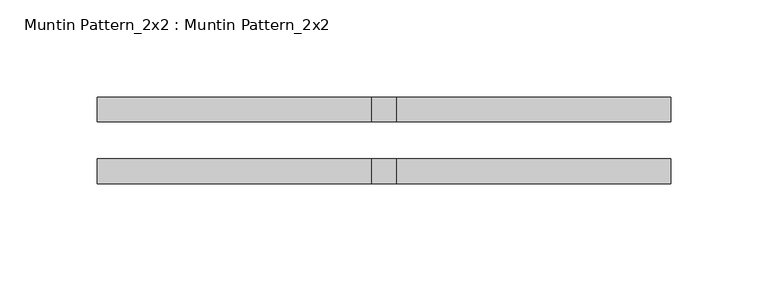
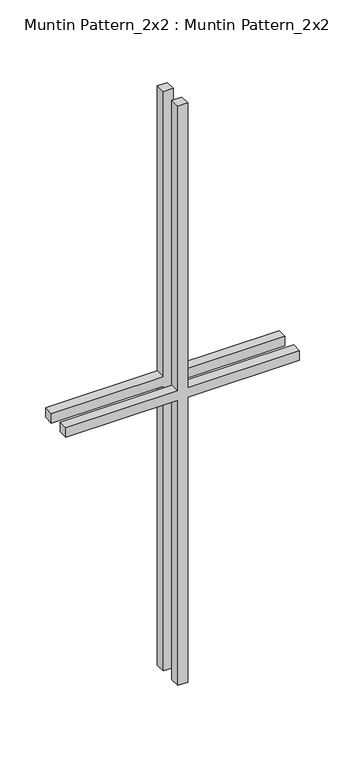
"""IFC4 building model written with IfcOpenShell, lengths in millimetres: proxy geometry, Muntin Pattern_2x2 : Muntin Pattern_2x2."""

from ifc_helpers import new_model, si_unit, frame, origin, place, context, project, spatial, polyline, outline, extrude, source, transform, mapped, element, save


def muntin_pattern_2x2_muntin_pattern_2x2_b3fe6957(model_context):
    return source(origin(), model_context, "Body", "SweptSolid", [
        extrude(outline(polyline([(393.7, -6.35), (393.7, -147.6375), (381.0, -147.6375), (381.0, -6.35), (0.0, -6.35), (0.0, 6.35), (381.0, 6.35), (381.0, 147.6375), (393.7, 147.6375), (393.7, 6.35), (774.7, 6.35), (774.7, -6.35), (393.7, -6.35)])), frame((0.0, 9.525, 0.0), z_axis=(0.0, 1.0, 0.0), x_axis=(0.0, 0.0, 1.0)), (0.0, 0.0, 1.0), 12.7),
        extrude(outline(polyline([(393.7, -6.35), (393.7, -147.6375), (381.0, -147.6375), (381.0, -6.35), (0.0, -6.35), (0.0, 6.35), (381.0, 6.35), (381.0, 147.6375), (393.7, 147.6375), (393.7, 6.35), (774.7, 6.35), (774.7, -6.35), (393.7, -6.35)])), frame((0.0, -22.225, 0.0), z_axis=(0.0, 1.0, 0.0), x_axis=(0.0, 0.0, 1.0)), (0.0, 0.0, 1.0), 12.7),
    ])


if __name__ == "__main__":
    model = new_model("IFC4")
    model_context = context("Model", 3, world=origin())
    ifc_project = project(units=[si_unit("LENGTHUNIT", "METRE", prefix="MILLI")], contexts=[model_context])
    site = spatial("IfcSite", under=ifc_project)
    building = spatial("IfcBuilding", under=site)
    placement = place(None, origin())
    muntin_pattern_2x2_muntin_pattern_2x2_shape = muntin_pattern_2x2_muntin_pattern_2x2_b3fe6957(model_context)
    element("IfcBuildingElementProxy", 1, Name="Muntin Pattern_2x2 : Muntin Pattern_2x2", ObjectType="Muntin Pattern_2x2 : Muntin Pattern_2x2", at=placement, inside=building, context=model_context, shape_type="MappedRepresentation", body=[
        mapped(muntin_pattern_2x2_muntin_pattern_2x2_shape, transform((0.0, 0.0, 0.0), x_axis=(1.0, 0.0, 0.0), y_axis=(0.0, 1.0, 0.0), z_axis=(0.0, 0.0, 1.0))),
    ])
    save(model, "model.ifc")

# Revit data of these elements
# Type "Muntin Pattern_2x2 : Muntin Pattern_2x2"
#   Width [instance default] = 48"
#   Thickness = 0.5"
#   Height [instance default] = 48"
#   Distance = 0.75"
#   Interior Material [instance default] = none
#   Exterior Material [instance default] = none
#   Default Elevation = 0
# Element 1 (IfcBuildingElementProxy, "Muntin Pattern_2x2 : Muntin Pattern_2x2")
#   Width = 11.625"
#   Height = 30.5"
#   Interior Material = Wood - Stained
#   Exterior Material = Clad - White
#   Materials on its faces: "Clad - White", "Wood - Stained"
# Materials
#   "Clad - White": class "Wood", colour RGB 242 242 238, transparency 0, Cost = 0
#   "Wood - Stained": class "Wood", colour RGB 224 178 126, transparency 0, Cost = 0
